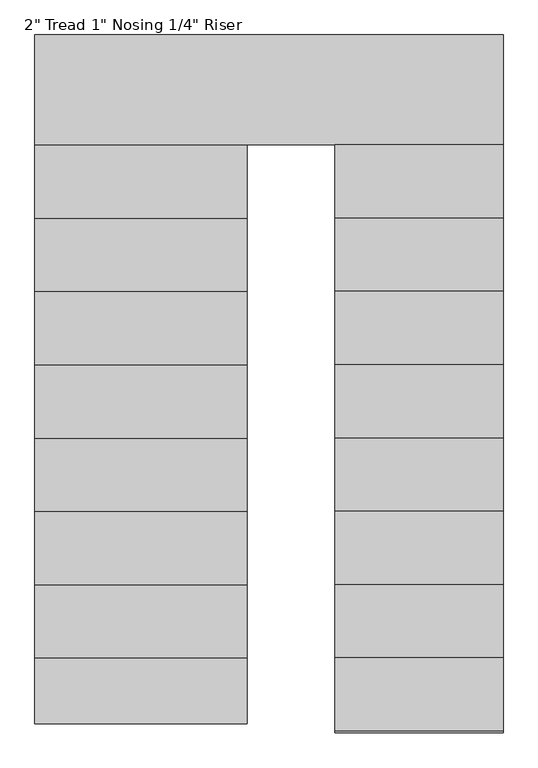
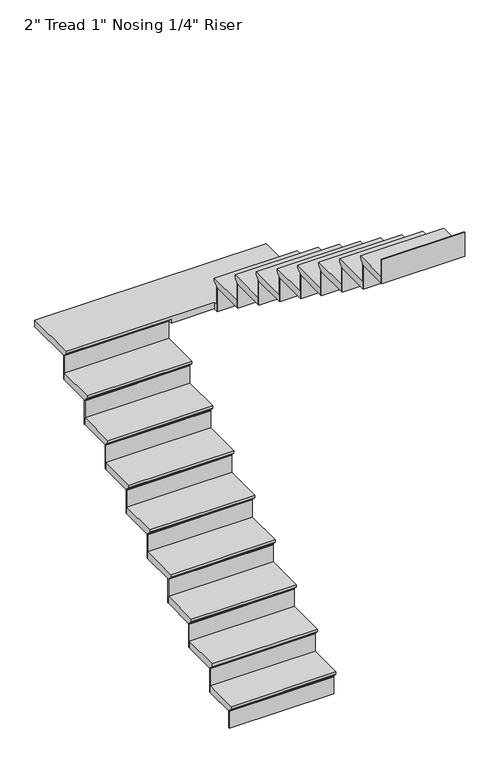
"""IFC4 building model written with IfcOpenShell, lengths in millimetres: stair flight geometry."""

from ifc_helpers import new_model, si_unit, origin, place, context, project, spatial, faceted_brep, source, transform, mapped, element, save


def stair_flight_1dbbfd26(model_context):
    return source(origin(), model_context, "Body", "Brep", [
        faceted_brep([(3394.0891134, -7650.9822004, 3359.15), (3394.0891134, -7650.9822004, 3378.2), (2657.4891134, -7650.9822004, 3378.2), (2657.4891134, -7650.9822004, 3359.15), (3394.0891134, -7625.5822004, 3333.75), (2657.4891134, -7625.5822004, 3333.75), (3394.0891134, -7396.9822004, 3378.2), (2657.4891134, -7396.9822004, 3378.2), (2657.4891134, -7625.5822004, 3327.4), (2657.4891134, -7396.9822004, 3327.4), (3394.0891134, -7396.9822004, 3327.4), (3394.0891134, -7625.5822004, 3327.4)], [[[0, 1, 2, 3]], [[4, 0, 3, 5]], [[2, 1, 6, 7]], [[8, 9, 10, 11]], [[2, 7, 9, 8, 5, 3]], [[8, 11, 4, 5]], [[6, 1, 0, 4, 11, 10]], [[7, 6, 10, 9]]]),
        faceted_brep([(3394.0891134, -7625.5822004, 3327.4), (3394.0891134, -7625.5822004, 3200.4), (3394.0891134, -7619.2322004, 3200.4), (3394.0891134, -7619.2322004, 3327.4), (2657.4891134, -7625.5822004, 3327.4), (2657.4891134, -7619.2322004, 3327.4), (2657.4891134, -7619.2322004, 3200.4), (2657.4891134, -7625.5822004, 3200.4)], [[[0, 1, 2, 3]], [[4, 5, 6, 7]], [[1, 0, 4, 7]], [[2, 1, 7, 6]], [[3, 2, 6, 5]], [[0, 3, 5, 4]]]),
        faceted_brep([(3394.0891134, -7396.9822004, 3505.2), (3394.0891134, -7396.9822004, 3327.4), (3394.0891134, -7390.6322004, 3327.4), (3394.0891134, -7390.6322004, 3505.2), (2657.4891134, -7396.9822004, 3505.2), (2657.4891134, -7390.6322004, 3505.2), (2657.4891134, -7390.6322004, 3327.4), (2657.4891134, -7396.9822004, 3327.4)], [[[0, 1, 2, 3]], [[4, 5, 6, 7]], [[1, 0, 4, 7]], [[2, 1, 7, 6]], [[3, 2, 6, 5]], [[0, 3, 5, 4]]]),
        faceted_brep([(2657.4891134, -7422.3822004, 3556.0), (3394.0891134, -7422.3822004, 3556.0), (3394.0891134, -7142.9822004, 3556.0), (2657.4891134, -7142.9822004, 3556.0), (2657.4891134, -7396.9822004, 3505.2), (2657.4891134, -7142.9822004, 3505.2), (3394.0891134, -7142.9822004, 3505.2), (3394.0891134, -7396.9822004, 3505.2), (2657.4891134, -7396.9822004, 3511.55), (2657.4891134, -7422.3822004, 3536.95), (3394.0891134, -7396.9822004, 3511.55), (3394.0891134, -7422.3822004, 3536.95)], [[[0, 1, 2, 3]], [[4, 5, 6, 7]], [[0, 3, 5, 4, 8, 9]], [[4, 7, 10, 8]], [[2, 1, 11, 10, 7, 6]], [[3, 2, 6, 5]], [[11, 1, 0, 9]], [[10, 11, 9, 8]]]),
        faceted_brep([(3394.0891134, -7142.9822004, 3683.0), (3394.0891134, -7142.9822004, 3505.2), (3394.0891134, -7136.6322004, 3505.2), (3394.0891134, -7136.6322004, 3683.0), (2657.4891134, -7142.9822004, 3683.0), (2657.4891134, -7136.6322004, 3683.0), (2657.4891134, -7136.6322004, 3505.2), (2657.4891134, -7142.9822004, 3505.2)], [[[0, 1, 2, 3]], [[4, 5, 6, 7]], [[1, 0, 4, 7]], [[2, 1, 7, 6]], [[3, 2, 6, 5]], [[0, 3, 5, 4]]]),
        faceted_brep([(2657.4891134, -7168.3822004, 3733.8), (3394.0891134, -7168.3822004, 3733.8), (3394.0891134, -6888.9822004, 3733.8), (2657.4891134, -6888.9822004, 3733.8), (2657.4891134, -7142.9822004, 3683.0), (2657.4891134, -6888.9822004, 3683.0), (3394.0891134, -6888.9822004, 3683.0), (3394.0891134, -7142.9822004, 3683.0), (2657.4891134, -7142.9822004, 3689.35), (2657.4891134, -7168.3822004, 3714.75), (3394.0891134, -7142.9822004, 3689.35), (3394.0891134, -7168.3822004, 3714.75)], [[[0, 1, 2, 3]], [[4, 5, 6, 7]], [[0, 3, 5, 4, 8, 9]], [[4, 7, 10, 8]], [[2, 1, 11, 10, 7, 6]], [[3, 2, 6, 5]], [[11, 1, 0, 9]], [[10, 11, 9, 8]]]),
        faceted_brep([(3394.0891134, -6888.9822004, 3860.8), (3394.0891134, -6888.9822004, 3683.0), (3394.0891134, -6882.6322004, 3683.0), (3394.0891134, -6882.6322004, 3860.8), (2657.4891134, -6888.9822004, 3860.8), (2657.4891134, -6882.6322004, 3860.8), (2657.4891134, -6882.6322004, 3683.0), (2657.4891134, -6888.9822004, 3683.0)], [[[0, 1, 2, 3]], [[4, 5, 6, 7]], [[1, 0, 4, 7]], [[2, 1, 7, 6]], [[3, 2, 6, 5]], [[0, 3, 5, 4]]]),
        faceted_brep([(2657.4891134, -6914.3822004, 3911.6), (3394.0891134, -6914.3822004, 3911.6), (3394.0891134, -6634.9822004, 3911.6), (2657.4891134, -6634.9822004, 3911.6), (2657.4891134, -6888.9822004, 3860.8), (2657.4891134, -6634.9822004, 3860.8), (3394.0891134, -6634.9822004, 3860.8), (3394.0891134, -6888.9822004, 3860.8), (2657.4891134, -6888.9822004, 3867.15), (2657.4891134, -6914.3822004, 3892.55), (3394.0891134, -6888.9822004, 3867.15), (3394.0891134, -6914.3822004, 3892.55)], [[[0, 1, 2, 3]], [[4, 5, 6, 7]], [[0, 3, 5, 4, 8, 9]], [[4, 7, 10, 8]], [[2, 1, 11, 10, 7, 6]], [[3, 2, 6, 5]], [[11, 1, 0, 9]], [[10, 11, 9, 8]]]),
        faceted_brep([(3394.0891134, -6634.9822004, 4038.6), (3394.0891134, -6634.9822004, 3860.8), (3394.0891134, -6628.6322004, 3860.8), (3394.0891134, -6628.6322004, 4038.6), (2657.4891134, -6634.9822004, 4038.6), (2657.4891134, -6628.6322004, 4038.6), (2657.4891134, -6628.6322004, 3860.8), (2657.4891134, -6634.9822004, 3860.8)], [[[0, 1, 2, 3]], [[4, 5, 6, 7]], [[1, 0, 4, 7]], [[2, 1, 7, 6]], [[3, 2, 6, 5]], [[0, 3, 5, 4]]]),
        faceted_brep([(2657.4891134, -6660.3822004, 4089.4), (3394.0891134, -6660.3822004, 4089.4), (3394.0891134, -6380.9822004, 4089.4), (2657.4891134, -6380.9822004, 4089.4), (2657.4891134, -6634.9822004, 4038.6), (2657.4891134, -6380.9822004, 4038.6), (3394.0891134, -6380.9822004, 4038.6), (3394.0891134, -6634.9822004, 4038.6), (2657.4891134, -6634.9822004, 4044.95), (2657.4891134, -6660.3822004, 4070.35), (3394.0891134, -6634.9822004, 4044.95), (3394.0891134, -6660.3822004, 4070.35)], [[[0, 1, 2, 3]], [[4, 5, 6, 7]], [[0, 3, 5, 4, 8, 9]], [[4, 7, 10, 8]], [[2, 1, 11, 10, 7, 6]], [[3, 2, 6, 5]], [[11, 1, 0, 9]], [[10, 11, 9, 8]]]),
        faceted_brep([(3394.0891134, -6380.9822004, 4216.4), (3394.0891134, -6380.9822004, 4038.6), (3394.0891134, -6374.6322004, 4038.6), (3394.0891134, -6374.6322004, 4216.4), (2657.4891134, -6380.9822004, 4216.4), (2657.4891134, -6374.6322004, 4216.4), (2657.4891134, -6374.6322004, 4038.6), (2657.4891134, -6380.9822004, 4038.6)], [[[0, 1, 2, 3]], [[4, 5, 6, 7]], [[1, 0, 4, 7]], [[2, 1, 7, 6]], [[3, 2, 6, 5]], [[0, 3, 5, 4]]]),
        faceted_brep([(2657.4891134, -6406.3822004, 4267.2), (3394.0891134, -6406.3822004, 4267.2), (3394.0891134, -6126.9822004, 4267.2), (2657.4891134, -6126.9822004, 4267.2), (2657.4891134, -6380.9822004, 4216.4), (2657.4891134, -6126.9822004, 4216.4), (3394.0891134, -6126.9822004, 4216.4), (3394.0891134, -6380.9822004, 4216.4), (2657.4891134, -6380.9822004, 4222.75), (2657.4891134, -6406.3822004, 4248.15), (3394.0891134, -6380.9822004, 4222.75), (3394.0891134, -6406.3822004, 4248.15)], [[[0, 1, 2, 3]], [[4, 5, 6, 7]], [[0, 3, 5, 4, 8, 9]], [[4, 7, 10, 8]], [[2, 1, 11, 10, 7, 6]], [[3, 2, 6, 5]], [[11, 1, 0, 9]], [[10, 11, 9, 8]]]),
        faceted_brep([(3394.0891134, -6126.9822004, 4394.2), (3394.0891134, -6126.9822004, 4216.4), (3394.0891134, -6120.6322004, 4216.4), (3394.0891134, -6120.6322004, 4394.2), (2657.4891134, -6126.9822004, 4394.2), (2657.4891134, -6120.6322004, 4394.2), (2657.4891134, -6120.6322004, 4216.4), (2657.4891134, -6126.9822004, 4216.4)], [[[0, 1, 2, 3]], [[4, 5, 6, 7]], [[1, 0, 4, 7]], [[2, 1, 7, 6]], [[3, 2, 6, 5]], [[0, 3, 5, 4]]]),
        faceted_brep([(2657.4891134, -6152.3822004, 4445.0), (3394.0891134, -6152.3822004, 4445.0), (3394.0891134, -5872.9822004, 4445.0), (2657.4891134, -5872.9822004, 4445.0), (2657.4891134, -6126.9822004, 4394.2), (2657.4891134, -5872.9822004, 4394.2), (3394.0891134, -5872.9822004, 4394.2), (3394.0891134, -6126.9822004, 4394.2), (2657.4891134, -6126.9822004, 4400.55), (2657.4891134, -6152.3822004, 4425.95), (3394.0891134, -6126.9822004, 4400.55), (3394.0891134, -6152.3822004, 4425.95)], [[[0, 1, 2, 3]], [[4, 5, 6, 7]], [[0, 3, 5, 4, 8, 9]], [[4, 7, 10, 8]], [[2, 1, 11, 10, 7, 6]], [[3, 2, 6, 5]], [[11, 1, 0, 9]], [[10, 11, 9, 8]]]),
        faceted_brep([(3394.0891134, -5872.9822004, 4572.0), (3394.0891134, -5872.9822004, 4394.2), (3394.0891134, -5866.6322004, 4394.2), (3394.0891134, -5866.6322004, 4572.0), (2657.4891134, -5872.9822004, 4572.0), (2657.4891134, -5866.6322004, 4572.0), (2657.4891134, -5866.6322004, 4394.2), (2657.4891134, -5872.9822004, 4394.2)], [[[0, 1, 2, 3]], [[4, 5, 6, 7]], [[1, 0, 4, 7]], [[2, 1, 7, 6]], [[3, 2, 6, 5]], [[0, 3, 5, 4]]]),
        faceted_brep([(2657.4891134, -5898.3822004, 4622.8), (3394.0891134, -5898.3822004, 4622.8), (3394.0891134, -5618.9822004, 4622.8), (2657.4891134, -5618.9822004, 4622.8), (2657.4891134, -5872.9822004, 4572.0), (2657.4891134, -5618.9822004, 4572.0), (3394.0891134, -5618.9822004, 4572.0), (3394.0891134, -5872.9822004, 4572.0), (2657.4891134, -5872.9822004, 4578.35), (2657.4891134, -5898.3822004, 4603.75), (3394.0891134, -5872.9822004, 4578.35), (3394.0891134, -5898.3822004, 4603.75)], [[[0, 1, 2, 3]], [[4, 5, 6, 7]], [[0, 3, 5, 4, 8, 9]], [[4, 7, 10, 8]], [[2, 1, 11, 10, 7, 6]], [[3, 2, 6, 5]], [[11, 1, 0, 9]], [[10, 11, 9, 8]]]),
        faceted_brep([(3394.0891134, -5618.9822004, 4749.8), (3394.0891134, -5618.9822004, 4572.0), (3394.0891134, -5612.6322004, 4572.0), (3394.0891134, -5612.6322004, 4749.8), (2657.4891134, -5618.9822004, 4749.8), (2657.4891134, -5612.6322004, 4749.8), (2657.4891134, -5612.6322004, 4572.0), (2657.4891134, -5618.9822004, 4572.0)], [[[0, 1, 2, 3]], [[4, 5, 6, 7]], [[1, 0, 4, 7]], [[2, 1, 7, 6]], [[3, 2, 6, 5]], [[0, 3, 5, 4]]]),
        faceted_brep([(4281.7311655, -5669.7822004, 4800.6), (4281.7311655, -5263.3822004, 4800.6), (2657.4891134, -5263.3822004, 4800.6), (2657.4891134, -5644.3822004, 4800.6), (3698.8891134, -5644.3822004, 4800.6), (3698.8891134, -5669.7822004, 4800.6), (4281.7311655, -5263.3822004, 4749.8), (4281.7311655, -5669.7822004, 4749.8), (3698.8891134, -5669.7822004, 4749.8), (3698.8891134, -5644.3822004, 4749.8), (3394.0891134, -5644.3822004, 4749.8), (3394.0891134, -5618.9822004, 4749.8), (2657.4891134, -5618.9822004, 4749.8), (2657.4891134, -5263.3822004, 4749.8), (3394.0891134, -5618.9822004, 4756.15), (2657.4891134, -5618.9822004, 4756.15), (2657.4891134, -5644.3822004, 4781.55), (3394.0891134, -5644.3822004, 4781.55)], [[[0, 1, 2, 3, 4, 5]], [[6, 7, 8, 9, 10, 11, 12, 13]], [[1, 0, 7, 6]], [[2, 1, 6, 13]], [[12, 11, 14, 15]], [[4, 3, 16, 17, 10, 9]], [[5, 4, 9, 8]], [[0, 5, 8, 7]], [[16, 15, 14, 17]], [[3, 2, 13, 12, 15, 16]], [[11, 10, 17, 14]]]),
        faceted_brep([(3698.8891134, -5669.7822004, 4927.6), (3698.8891134, -5669.7822004, 4749.8), (3698.8891134, -5676.1322004, 4749.8), (3698.8891134, -5676.1322004, 4927.6), (4281.7311655, -5669.7822004, 4927.6), (4281.7311655, -5676.1322004, 4927.6), (4281.7311655, -5676.1322004, 4749.8), (4281.7311655, -5669.7822004, 4749.8)], [[[0, 1, 2, 3]], [[4, 5, 6, 7]], [[1, 0, 4, 7]], [[2, 1, 7, 6]], [[3, 2, 6, 5]], [[0, 3, 5, 4]]]),
        faceted_brep([(4281.7311655, -5644.3822004, 4978.4), (3698.8891134, -5644.3822004, 4978.4), (3698.8891134, -5923.7822004, 4978.4), (4281.7311655, -5923.7822004, 4978.4), (4281.7311655, -5669.7822004, 4927.6), (4281.7311655, -5923.7822004, 4927.6), (3698.8891134, -5923.7822004, 4927.6), (3698.8891134, -5669.7822004, 4927.6), (4281.7311655, -5669.7822004, 4933.95), (4281.7311655, -5644.3822004, 4959.35), (3698.8891134, -5669.7822004, 4933.95), (3698.8891134, -5644.3822004, 4959.35)], [[[0, 1, 2, 3]], [[4, 5, 6, 7]], [[0, 3, 5, 4, 8, 9]], [[4, 7, 10, 8]], [[2, 1, 11, 10, 7, 6]], [[3, 2, 6, 5]], [[11, 1, 0, 9]], [[10, 11, 9, 8]]]),
        faceted_brep([(3698.8891134, -5923.7822004, 5105.4), (3698.8891134, -5923.7822004, 4927.6), (3698.8891134, -5930.1322004, 4927.6), (3698.8891134, -5930.1322004, 5105.4), (4281.7311655, -5923.7822004, 5105.4), (4281.7311655, -5930.1322004, 5105.4), (4281.7311655, -5930.1322004, 4927.6), (4281.7311655, -5923.7822004, 4927.6)], [[[0, 1, 2, 3]], [[4, 5, 6, 7]], [[1, 0, 4, 7]], [[2, 1, 7, 6]], [[3, 2, 6, 5]], [[0, 3, 5, 4]]]),
        faceted_brep([(4281.7311655, -5898.3822004, 5156.2), (3698.8891134, -5898.3822004, 5156.2), (3698.8891134, -6177.7822004, 5156.2), (4281.7311655, -6177.7822004, 5156.2), (4281.7311655, -5923.7822004, 5105.4), (4281.7311655, -6177.7822004, 5105.4), (3698.8891134, -6177.7822004, 5105.4), (3698.8891134, -5923.7822004, 5105.4), (4281.7311655, -5923.7822004, 5111.75), (4281.7311655, -5898.3822004, 5137.15), (3698.8891134, -5923.7822004, 5111.75), (3698.8891134, -5898.3822004, 5137.15)], [[[0, 1, 2, 3]], [[4, 5, 6, 7]], [[0, 3, 5, 4, 8, 9]], [[4, 7, 10, 8]], [[2, 1, 11, 10, 7, 6]], [[3, 2, 6, 5]], [[11, 1, 0, 9]], [[10, 11, 9, 8]]]),
        faceted_brep([(3698.8891134, -6177.7822004, 5283.2), (3698.8891134, -6177.7822004, 5105.4), (3698.8891134, -6184.1322004, 5105.4), (3698.8891134, -6184.1322004, 5283.2), (4281.7311655, -6177.7822004, 5283.2), (4281.7311655, -6184.1322004, 5283.2), (4281.7311655, -6184.1322004, 5105.4), (4281.7311655, -6177.7822004, 5105.4)], [[[0, 1, 2, 3]], [[4, 5, 6, 7]], [[1, 0, 4, 7]], [[2, 1, 7, 6]], [[3, 2, 6, 5]], [[0, 3, 5, 4]]]),
        faceted_brep([(4281.7311655, -6152.3822004, 5334.0), (3698.8891134, -6152.3822004, 5334.0), (3698.8891134, -6431.7822004, 5334.0), (4281.7311655, -6431.7822004, 5334.0), (4281.7311655, -6177.7822004, 5283.2), (4281.7311655, -6431.7822004, 5283.2), (3698.8891134, -6431.7822004, 5283.2), (3698.8891134, -6177.7822004, 5283.2), (4281.7311655, -6177.7822004, 5289.55), (4281.7311655, -6152.3822004, 5314.95), (3698.8891134, -6177.7822004, 5289.55), (3698.8891134, -6152.3822004, 5314.95)], [[[0, 1, 2, 3]], [[4, 5, 6, 7]], [[0, 3, 5, 4, 8, 9]], [[4, 7, 10, 8]], [[2, 1, 11, 10, 7, 6]], [[3, 2, 6, 5]], [[11, 1, 0, 9]], [[10, 11, 9, 8]]]),
        faceted_brep([(3698.8891134, -6431.7822004, 5461.0), (3698.8891134, -6431.7822004, 5283.2), (3698.8891134, -6438.1322004, 5283.2), (3698.8891134, -6438.1322004, 5461.0), (4281.7311655, -6431.7822004, 5461.0), (4281.7311655, -6438.1322004, 5461.0), (4281.7311655, -6438.1322004, 5283.2), (4281.7311655, -6431.7822004, 5283.2)], [[[0, 1, 2, 3]], [[4, 5, 6, 7]], [[1, 0, 4, 7]], [[2, 1, 7, 6]], [[3, 2, 6, 5]], [[0, 3, 5, 4]]]),
        faceted_brep([(4281.7311655, -6406.3822004, 5511.8), (3698.8891134, -6406.3822004, 5511.8), (3698.8891134, -6685.7822004, 5511.8), (4281.7311655, -6685.7822004, 5511.8), (4281.7311655, -6431.7822004, 5461.0), (4281.7311655, -6685.7822004, 5461.0), (3698.8891134, -6685.7822004, 5461.0), (3698.8891134, -6431.7822004, 5461.0), (4281.7311655, -6431.7822004, 5467.35), (4281.7311655, -6406.3822004, 5492.75), (3698.8891134, -6431.7822004, 5467.35), (3698.8891134, -6406.3822004, 5492.75)], [[[0, 1, 2, 3]], [[4, 5, 6, 7]], [[0, 3, 5, 4, 8, 9]], [[4, 7, 10, 8]], [[2, 1, 11, 10, 7, 6]], [[3, 2, 6, 5]], [[11, 1, 0, 9]], [[10, 11, 9, 8]]]),
        faceted_brep([(3698.8891134, -6685.7822004, 5638.8), (3698.8891134, -6685.7822004, 5461.0), (3698.8891134, -6692.1322004, 5461.0), (3698.8891134, -6692.1322004, 5638.8), (4281.7311655, -6685.7822004, 5638.8), (4281.7311655, -6692.1322004, 5638.8), (4281.7311655, -6692.1322004, 5461.0), (4281.7311655, -6685.7822004, 5461.0)], [[[0, 1, 2, 3]], [[4, 5, 6, 7]], [[1, 0, 4, 7]], [[2, 1, 7, 6]], [[3, 2, 6, 5]], [[0, 3, 5, 4]]]),
        faceted_brep([(4281.7311655, -6660.3822004, 5689.6), (3698.8891134, -6660.3822004, 5689.6), (3698.8891134, -6939.7822004, 5689.6), (4281.7311655, -6939.7822004, 5689.6), (4281.7311655, -6685.7822004, 5638.8), (4281.7311655, -6939.7822004, 5638.8), (3698.8891134, -6939.7822004, 5638.8), (3698.8891134, -6685.7822004, 5638.8), (4281.7311655, -6685.7822004, 5645.15), (4281.7311655, -6660.3822004, 5670.55), (3698.8891134, -6685.7822004, 5645.15), (3698.8891134, -6660.3822004, 5670.55)], [[[0, 1, 2, 3]], [[4, 5, 6, 7]], [[0, 3, 5, 4, 8, 9]], [[4, 7, 10, 8]], [[2, 1, 11, 10, 7, 6]], [[3, 2, 6, 5]], [[11, 1, 0, 9]], [[10, 11, 9, 8]]]),
        faceted_brep([(3698.8891134, -6939.7822004, 5816.6), (3698.8891134, -6939.7822004, 5638.8), (3698.8891134, -6946.1322004, 5638.8), (3698.8891134, -6946.1322004, 5816.6), (4281.7311655, -6939.7822004, 5816.6), (4281.7311655, -6946.1322004, 5816.6), (4281.7311655, -6946.1322004, 5638.8), (4281.7311655, -6939.7822004, 5638.8)], [[[0, 1, 2, 3]], [[4, 5, 6, 7]], [[1, 0, 4, 7]], [[2, 1, 7, 6]], [[3, 2, 6, 5]], [[0, 3, 5, 4]]]),
        faceted_brep([(4281.7311655, -6914.3822004, 5867.4), (3698.8891134, -6914.3822004, 5867.4), (3698.8891134, -7193.7822004, 5867.4), (4281.7311655, -7193.7822004, 5867.4), (4281.7311655, -6939.7822004, 5816.6), (4281.7311655, -7193.7822004, 5816.6), (3698.8891134, -7193.7822004, 5816.6), (3698.8891134, -6939.7822004, 5816.6), (4281.7311655, -6939.7822004, 5822.95), (4281.7311655, -6914.3822004, 5848.35), (3698.8891134, -6939.7822004, 5822.95), (3698.8891134, -6914.3822004, 5848.35)], [[[0, 1, 2, 3]], [[4, 5, 6, 7]], [[0, 3, 5, 4, 8, 9]], [[4, 7, 10, 8]], [[2, 1, 11, 10, 7, 6]], [[3, 2, 6, 5]], [[11, 1, 0, 9]], [[10, 11, 9, 8]]]),
        faceted_brep([(3698.8891134, -7193.7822004, 5994.4), (3698.8891134, -7193.7822004, 5816.6), (3698.8891134, -7200.1322004, 5816.6), (3698.8891134, -7200.1322004, 5994.4), (4281.7311655, -7193.7822004, 5994.4), (4281.7311655, -7200.1322004, 5994.4), (4281.7311655, -7200.1322004, 5816.6), (4281.7311655, -7193.7822004, 5816.6)], [[[0, 1, 2, 3]], [[4, 5, 6, 7]], [[1, 0, 4, 7]], [[2, 1, 7, 6]], [[3, 2, 6, 5]], [[0, 3, 5, 4]]]),
        faceted_brep([(4281.7311655, -7168.3822004, 6045.2), (3698.8891134, -7168.3822004, 6045.2), (3698.8891134, -7447.7822004, 6045.2), (4281.7311655, -7447.7822004, 6045.2), (4281.7311655, -7193.7822004, 5994.4), (4281.7311655, -7447.7822004, 5994.4), (3698.8891134, -7447.7822004, 5994.4), (3698.8891134, -7193.7822004, 5994.4), (4281.7311655, -7193.7822004, 6000.75), (4281.7311655, -7168.3822004, 6026.15), (3698.8891134, -7193.7822004, 6000.75), (3698.8891134, -7168.3822004, 6026.15)], [[[0, 1, 2, 3]], [[4, 5, 6, 7]], [[0, 3, 5, 4, 8, 9]], [[4, 7, 10, 8]], [[2, 1, 11, 10, 7, 6]], [[3, 2, 6, 5]], [[11, 1, 0, 9]], [[10, 11, 9, 8]]]),
        faceted_brep([(3698.8891134, -7447.7822004, 6172.2), (3698.8891134, -7447.7822004, 5994.4), (3698.8891134, -7454.1322004, 5994.4), (3698.8891134, -7454.1322004, 6172.2), (4281.7311655, -7447.7822004, 6172.2), (4281.7311655, -7454.1322004, 6172.2), (4281.7311655, -7454.1322004, 5994.4), (4281.7311655, -7447.7822004, 5994.4)], [[[0, 1, 2, 3]], [[4, 5, 6, 7]], [[1, 0, 4, 7]], [[2, 1, 7, 6]], [[3, 2, 6, 5]], [[0, 3, 5, 4]]]),
        faceted_brep([(3698.8891134, -7676.3822004, 6350.0), (3698.8891134, -7676.3822004, 6172.2), (3698.8891134, -7682.7322004, 6172.2), (3698.8891134, -7682.7322004, 6350.0), (4281.7311655, -7676.3822004, 6350.0), (4281.7311655, -7682.7322004, 6350.0), (4281.7311655, -7682.7322004, 6172.2), (4281.7311655, -7676.3822004, 6172.2)], [[[0, 1, 2, 3]], [[4, 5, 6, 7]], [[1, 0, 4, 7]], [[2, 1, 7, 6]], [[3, 2, 6, 5]], [[0, 3, 5, 4]]]),
        faceted_brep([(4281.7311655, -7422.3822004, 6223.0), (3698.8891134, -7422.3822004, 6223.0), (3698.8891134, -7676.3822004, 6223.0), (4281.7311655, -7676.3822004, 6223.0), (4281.7311655, -7447.7822004, 6172.2), (4281.7311655, -7676.3822004, 6172.2), (3698.8891134, -7676.3822004, 6172.2), (3698.8891134, -7447.7822004, 6172.2), (4281.7311655, -7447.7822004, 6178.55), (4281.7311655, -7422.3822004, 6203.95), (3698.8891134, -7447.7822004, 6178.55), (3698.8891134, -7422.3822004, 6203.95)], [[[0, 1, 2, 3]], [[4, 5, 6, 7]], [[0, 3, 5, 4, 8, 9]], [[4, 7, 10, 8]], [[2, 1, 11, 10, 7, 6]], [[3, 2, 6, 5]], [[11, 1, 0, 9]], [[10, 11, 9, 8]]]),
    ])


if __name__ == "__main__":
    model = new_model("IFC4")
    model_context = context("Model", 3, world=origin())
    ifc_project = project(units=[si_unit("LENGTHUNIT", "METRE", prefix="MILLI")], contexts=[model_context])
    site = spatial("IfcSite", under=ifc_project)
    building = spatial("IfcBuilding", under=site)
    placement = place(None, origin())
    stair_flight_shape = stair_flight_1dbbfd26(model_context)
    element("IfcStairFlight", 1, ObjectType="2\" Tread 1\" Nosing 1/4\" Riser", at=placement, inside=building, context=model_context, shape_type="MappedRepresentation", body=[
        mapped(stair_flight_shape, transform((0.0, 0.0, 0.0), x_axis=(1.0, 0.0, 0.0), y_axis=(0.0, 1.0, 0.0), z_axis=(0.0, 0.0, 1.0))),
    ])
    save(model, "model.ifc")
